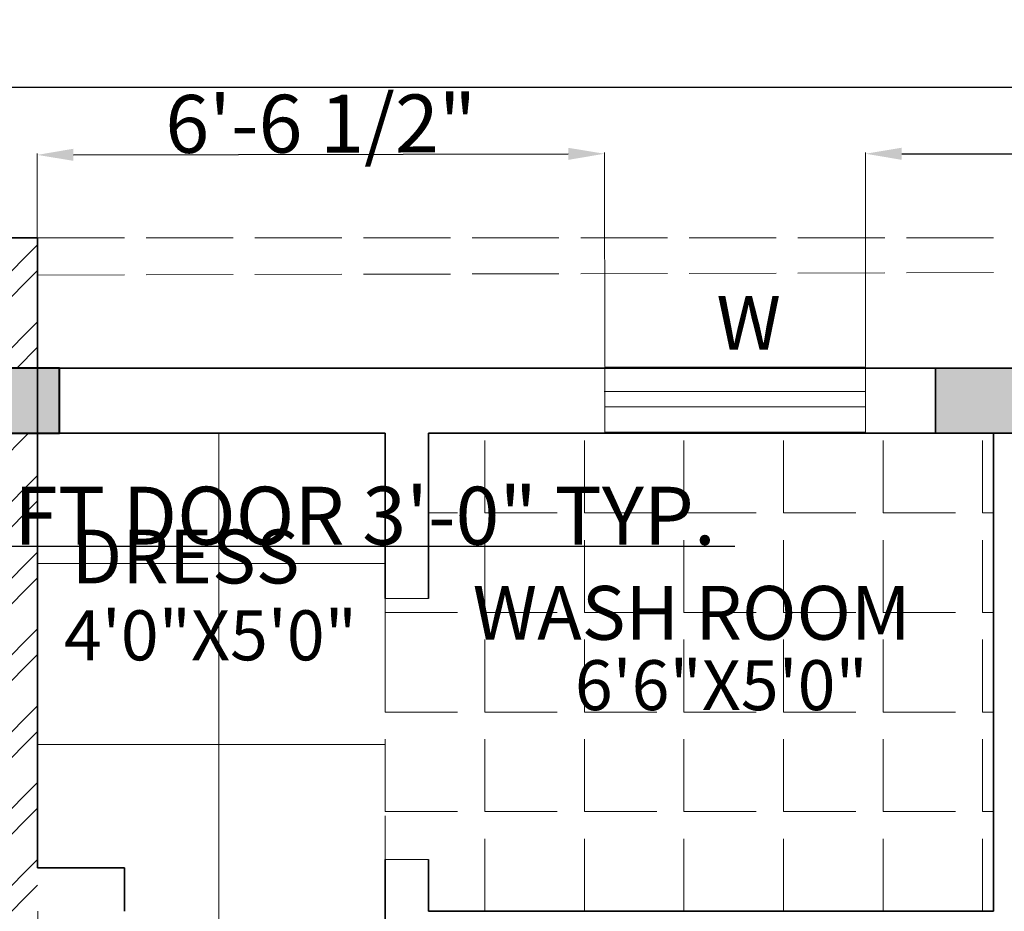
# Model space of a CAD drawing. Units: inches. Extents: x 351 to 1738, y -265 to 286.
# Tile 27 of 38: x 1110 to 1246, y 163 to 286. Entities that reach past the tile are written whole.
import ezdxf

# ---------------------------------------------------------------- set-up
doc = ezdxf.new("R2010")
doc.units = ezdxf.units.IN
doc.header["$MEASUREMENT"] = 0
doc.linetypes.add('ACAD_ISO02W100', pattern=[15, 12, -3])
doc.linetypes.add('ACAD_ISO03W100', pattern=[30, 12, -18])
for name, color, linetype, lineweight in [('A-ANNO-DIMS', 2, 'Continuous', 18), ('A-ANNO-SYMB', 7, 'Continuous', 18), ('A-AREA-IDEN', 7, 'Continuous', 18), ('A-COLS', 7, 'Continuous', 40), ('A-COLS-PATT', 6, 'Continuous', 13), ('A-DOOR', 3, 'Continuous', 18), ('A-DOOR-HIDN', 3, 'ACAD_ISO03W100', 13), ('A-FLOR-OVHD', 1, 'ACAD_ISO02W100', 18), ('A-FLOR-PATT', 9, 'Continuous', 9), ('A-GLAZ', 4, 'Continuous', 18), ('A-WALL', 7, 'Continuous', 35), ('A-WALL-PATT', 152, 'Continuous', 13)]:
    doc.layers.add(name, color=color, linetype=linetype, lineweight=lineweight)
doc.styles.add('Annotative', font='arial.ttf')
doc.styles.get("Standard").update_dxf_attribs({"font": 'arial.ttf'})
doc.dimstyles.get("Standard").update_dxf_attribs({"dimtxt": 8, "dimasz": 5, "dimexe": 0.18, "dimexo": 0.0625, "dimgap": 0.09, "dimtad": 1, "dimtoh": 1, "dimzin": 0, "dimdsep": 46, "dimlunit": 4, "dimtxsty": 'Standard', "dimcen": 0, "dimclre": 256, "dimadec": 0, "dimazin": 0, "dimtfac": 1, "dimtofl": 0, "dimtmove": 0, "dimatfit": 3, "dimfxl": 1, "dimtolj": 1, "dimtzin": 0, "dimlwe": -1, "dimarcsym": 0})

# ---------------------------------------------------------------- blocks, each defined once
blk = doc.blocks.new('*D7')
at = {"layer": 'A-ANNO-DIMS', "color": 0, "transparency": 16777216}
for p, q in [((1034.7, 256.03), (1034.7, 276.92)), ((1566.7, 256.03), (1566.7, 276.92))]:
    blk.add_line(p, q, dxfattribs=at)
at = {"layer": 'A-ANNO-DIMS', "color": 0, "lineweight": -2, "transparency": 16777216}
blk.add_line((1039.7, 276.74), (1561.7, 276.74), dxfattribs=at)
at = {"layer": 'A-ANNO-DIMS', "color": 0, "transparency": 16777216}
for points in [[(1039.7, 277.57), (1039.7, 275.91), (1034.7, 276.74)], [(1561.7, 277.57), (1561.7, 275.91), (1566.7, 276.74)]]:
    blk.add_solid(points, dxfattribs=at)
at = {"layer": 'Defpoints', "color": 0, "transparency": 16777216}
for p in [(1566.7, 276.74), (1034.7, 255.96), (1566.7, 255.96)]:
    blk.add_point(p, dxfattribs=at)
at = {"layer": 'A-ANNO-DIMS', "color": 0, "transparency": 16777216, "insert": (1300.7, 280.83), "char_height": 8, "attachment_point": 5}
blk.add_mtext('\\A1;44\'-4"', dxfattribs=at)
blk = doc.blocks.new('*D54')
at = {"layer": 'A-ANNO-DIMS', "transparency": 16777216}
for p, q in [((1056.7, 208.03), (1056.7, 213.54)), ((1092.7, 208.03), (1092.7, 213.54))]:
    blk.add_line(p, q, dxfattribs=at)
at = {"layer": 'A-ANNO-DIMS', "color": 0, "lineweight": -2, "transparency": 16777216}
for p, q in [((1061.7, 213.36), (1087.7, 213.36)), ((1092.7, 213.36), (1209.01, 213.36))]:
    blk.add_line(p, q, dxfattribs=at)
at = {"layer": 'A-ANNO-DIMS', "color": 0, "transparency": 16777216}
for points in [[(1061.7, 214.2), (1061.7, 212.53), (1056.7, 213.36)], [(1087.7, 214.2), (1087.7, 212.53), (1092.7, 213.36)]]:
    blk.add_solid(points, dxfattribs=at)
at = {"layer": 'Defpoints', "color": 0, "transparency": 16777216}
for p in [(1092.7, 213.36), (1056.7, 207.96), (1092.7, 207.96)]:
    blk.add_point(p, dxfattribs=at)
at = {"layer": 'A-ANNO-DIMS', "color": 0, "transparency": 16777216, "insert": (1153.35, 217.59), "char_height": 8, "attachment_point": 5}
blk.add_mtext('\\A1;LIFT DOOR 3\'-0" TYP.', dxfattribs=at)
blk = doc.blocks.new('*D62')
at = {"layer": 'A-ANNO-DIMS', "transparency": 16777216}
for p, q in [((1112.7, 238.03), (1112.65, 267.59)), ((1191.04, 238.18), (1190.98, 267.75))]:
    blk.add_line(p, q, dxfattribs=at)
at = {"layer": 'A-ANNO-DIMS', "color": 0, "lineweight": -2, "transparency": 16777216}
blk.add_line((1117.65, 267.42), (1185.98, 267.56), dxfattribs=at)
at = {"layer": 'A-ANNO-DIMS', "color": 0, "transparency": 16777216}
for points in [[(1117.65, 268.26), (1117.65, 266.59), (1112.65, 267.41)], [(1185.98, 268.39), (1185.98, 266.72), (1190.98, 267.57)]]:
    blk.add_solid(points, dxfattribs=at)
at = {"layer": 'Defpoints', "color": 0, "transparency": 16777216}
for p in [(1190.98, 267.57), (1191.04, 238.12), (1112.7, 237.96)]:
    blk.add_point(p, dxfattribs=at)
at = {"layer": 'A-ANNO-DIMS', "color": 0, "transparency": 16777216, "insert": (1151.81, 271.72), "char_height": 8, "attachment_point": 5, "rotation": 0.1116}
blk.add_mtext('\\A1;6\'-6 1/2"', dxfattribs=at)
blk = doc.blocks.new('*D63')
at = {"layer": 'A-ANNO-DIMS', "transparency": 16777216}
for p, q in [((1227.04, 238.18), (1227.04, 267.75)), ((1266.55, 238.18), (1266.55, 267.75))]:
    blk.add_line(p, q, dxfattribs=at)
at = {"layer": 'A-ANNO-DIMS', "color": 0, "lineweight": -2, "transparency": 16777216}
for p, q in [((1232.04, 267.57), (1261.55, 267.57)), ((1266.55, 267.57), (1311.63, 267.57))]:
    blk.add_line(p, q, dxfattribs=at)
at = {"layer": 'A-ANNO-DIMS', "color": 0, "transparency": 16777216}
for points in [[(1232.04, 268.4), (1232.04, 266.73), (1227.04, 267.57)], [(1261.55, 268.4), (1261.55, 266.73), (1266.55, 267.57)]]:
    blk.add_solid(points, dxfattribs=at)
at = {"layer": 'Defpoints', "color": 0, "transparency": 16777216}
for p in [(1266.55, 267.57), (1227.04, 238.12), (1266.55, 238.12)]:
    blk.add_point(p, dxfattribs=at)
at = {"layer": 'A-ANNO-DIMS', "color": 0, "transparency": 16777216, "insert": (1291.59, 271.79), "char_height": 8, "attachment_point": 5}
blk.add_mtext('\\A1;3\'-3 1/2"', dxfattribs=at)

msp = doc.modelspace()

# ---------------------------------------------------------------- hatches: boundary and pattern name
at = {"layer": 'A-COLS-PATT'}
h = msp.add_hatch(color=256, dxfattribs=at)
h.dxf.hatch_style = 1
h.paths.add_polyline_path([(1112.704, 237.963), (1103.704, 237.963), (1103.704, 228.963), (1112.704, 228.963)])
h.paths.add_polyline_path([(1115.704, 237.963), (1112.704, 237.963), (1112.704, 228.963), (1115.704, 228.963)])
h.paths.add_polyline_path([(1043.704, 255.963), (1034.704, 255.963), (1034.704, 243.963), (1043.704, 243.963)])
h.paths.add_polyline_path([(1043.704, 210.963), (1034.704, 210.963), (1034.704, 198.963), (1043.704, 198.963)])
h.paths.add_polyline_path([(1043.704, -45.037), (1034.704, -45.037), (1034.704, -57.037), (1043.704, -57.037)])
h.paths.add_polyline_path([(1112.704, -45.037), (1103.704, -45.037), (1103.704, -57.037), (1112.704, -57.037)])
h.paths.add_polyline_path([(1112.704, -161.037), (1103.704, -161.037), (1103.704, -164.037), (1103.704, -173.037), (1112.704, -173.037)])
h.paths.add_polyline_path([(1043.704, -161.037), (1034.704, -161.037), (1034.704, -173.037), (1043.704, -173.037)])
h.paths.add_polyline_path([(1248.549, -164.037), (1236.549, -164.037), (1236.549, -173.037), (1248.549, -173.037)])
h.paths.add_polyline_path([(1248.549, -50), (1236.549, -50), (1236.549, -59), (1248.549, -59)])
h.paths.add_polyline_path([(1248.704, 73.463), (1244.704, 73.463), (1244.704, 64.463), (1248.704, 64.463)])
h.paths.add_polyline_path([(1244.704, 73.463), (1236.704, 73.463), (1236.704, 64.463), (1244.704, 64.463)])
h.paths.add_polyline_path([(1248.704, 237.963), (1236.704, 237.963), (1236.704, 228.963), (1248.704, 228.963)])
h.paths.add_polyline_path([(1392.204, 237.963), (1380.204, 237.963), (1380.204, 228.963), (1392.204, 228.963)])
h.paths.add_polyline_path([(1536.064, 237.963), (1524.064, 237.963), (1524.064, 228.963), (1536.064, 228.963)])
h.paths.add_polyline_path([(1536.064, 73.463), (1524.064, 73.463), (1524.064, 64.463), (1536.064, 64.463)])
h.paths.add_polyline_path([(1384.204, 73.463), (1380.204, 73.463), (1380.204, 64.463), (1384.204, 64.463)])
h.paths.add_polyline_path([(1392.064, 73.463), (1384.204, 73.463), (1384.204, 64.463), (1392.064, 64.463)])
h.paths.add_polyline_path([(1536.064, -53.037), (1524.064, -53.037), (1524.064, -57.037), (1536.064, -57.037)])
h.paths.add_polyline_path([(1536.064, -48.037), (1524.064, -48.037), (1524.064, -53.037), (1536.064, -53.037)])
h.paths.add_polyline_path([(1392.064, -48.037), (1380.064, -48.037), (1380.064, -56.5), (1380.065, -57.037), (1392.064, -57.037)])
h.paths.add_polyline_path([(1536.064, -164.037), (1524.064, -164.037), (1524.064, -173.037), (1536.064, -173.037)])
at = {"layer": 'A-FLOR-PATT', "transparency": 33554559}
h = msp.add_hatch(dxfattribs=at)
h.set_pattern_fill('ANSI37', color=256, scale=200, angle=135)
h.set_pattern_definition([(180, (1112.704, -164.037), (-2e-15, -25), []), (270, (1112.704, -164.037), (25, -5e-15), [])])
h.paths.add_polyline_path([(1380.064, 73.463), (1380.132, 148.463), (1338.064, 148.463), (1290.704, 148.463), (1290.704, 88.463), (1248.704, 88.463), (1248.704, -2.009), (1244.704, -2.009), (1244.704, 142.457), (1160.704, 142.457), (1160.704, 158.963), (1160.704, 170.137), (1160.704, 206.137), (1160.704, 228.963), (1112.704, 228.963), (1112.704, 209.963), (1112.704, 168.963), (1124.704, 168.963), (1124.704, 162.963), (1112.704, 162.963), (1112.704, 64.463), (1112.704, 60.463), (1112.704, 0.463), (1112.704, -48.026), (1146.804, -47.981), (1146.804, -35.691), (1207.804, -35.691), (1207.804, -47.902), (1236.542, -47.864), (1236.544, -50.009), (1248.5, -50.009), (1248.506, -102.915), (1248.512, -150.915), (1248.514, -164.037), (1248.549, -164.037), (1273.017, -164.037), (1273.017, -128.799), (1355.24, -128.799), (1355.24, -164.037), (1384.204, -164.037), (1384.204, -57.037), (1380.064, -57.037), (1380.064, -48.037), (1392.064, -48.037), (1392.064, -53.037), (1406.549, -53.037), (1406.549, -57.037), (1401.204, -57.037), (1401.204, -147.037), (1468.204, -147.037), (1468.204, -138.5), (1472.204, -138.5), (1472.204, -102.5), (1468.204, -102.5), (1468.204, -57.037), (1442.549, -57.037), (1442.549, -53.037), (1463.049, -53.037), (1463.049, -40.747), (1524.049, -40.747), (1524.049, -48.037), (1536.064, -48.037), (1536.064, -53.037), (1557.704, -53.037), (1557.704, 204.963), (1384.204, 204.963), (1384.204, 73.463), (1392.064, 73.463), (1392.064, 64.463), (1384.204, 64.463), (1384.204, -3.5), (1380.204, -3.537), (1380.204, 64.463), (1380.064, 64.463)])
h.paths.add_polyline_path([(1510.714, 86.458, -0.1039845), (1511.661, 85.595, 0.4704384), (1510.158, 87.614, 0.0961001)], flags=16)
h.paths.add_polyline_path([(1510.443, 100.266, 0.009798), (1504.693, 100.48, 0.0287898), (1504.6, 99.767, -0.1653311), (1505.519, 96.135, -0.1436014)], flags=16)
h.paths.add_polyline_path([(1487.201, 85.595, -0.1039845), (1488.148, 86.458, 0.0961001), (1488.704, 87.614, 0.4704384)], flags=0)
h.paths.add_polyline_path([(1495.052, 100.43), (1494.178, 100.43, -0.0264629), (1494.262, 99.774, -0.1442193)], flags=16)
h.paths.add_polyline_path([(1444.485, 86.458, -0.1039845), (1445.433, 85.595, 0.4704384), (1443.93, 87.614, 0.0961001)], flags=16)
h.paths.add_polyline_path([(1420.972, 85.595, -0.1039845), (1421.92, 86.458, 0.0961001), (1422.475, 87.614, 0.4704384)], flags=16)
h.paths.add_polyline_path([(1428.632, 100.335, 0.0010541), (1427.971, 100.309, -0.0215241), (1428.033, 99.774, -0.1143008)], flags=16)
h.paths.add_polyline_path([(1419.906, 143.708, 0.0249793), (1420.222, 157.526), (1421.573, 159.101), (1421.573, 175.369), (1391.393, 175.369), (1391.393, 200.519), (1542.294, 200.519), (1542.294, 175.369), (1512.028, 175.369, 0.0198653), (1511.521, 153.838, 0.0251335), (1512.758, 118.323, 0.0205529), (1512.942, 115.253), (1419.834, 115.253, -0.0004142), (1419.843, 124.798), (1413.059, 124.798), (1413.059, 84.437, -0.0618528), (1415.831, 80.45, -0.0930773), (1420.972, 85.595, -0.2675367), (1422.371, 84.732, 0.0851103), (1424.052, 84.616, -0.8853927), (1424.033, 84.851, -1.1258145), (1424.073, 84.366, -0.0879871), (1422.371, 84.732, -0.2675367), (1422.326, 83.089, -0.3705421), (1420.972, 85.595, 0.0930773), (1415.831, 80.45, -0.0874142), (1417.914, 73.937), (1418.941, 73.937, 0.0272504), (1418.913, 76.906, -0.1157032), (1421.051, 73.937), (1445.354, 73.937, -0.1157032), (1447.492, 76.906, 0.0272504), (1447.464, 73.937), (1448.491, 73.937, -0.0874142), (1450.574, 80.45, 0.0930773), (1445.433, 85.595, -0.3705421), (1444.079, 83.089, -0.2675367), (1444.034, 84.732, -0.0879871), (1442.332, 84.366, -1.1258145), (1442.372, 84.851, -2.0327363), (1442.364, 84.368, 0.0863779), (1444.034, 84.732, -0.2675367), (1445.433, 85.595, -0.0930773), (1450.574, 80.45, -0.2577317), (1466.483, 90.927, -0.4786702), (1468.832, 91.907, -0.4786702), (1471.18, 90.927, -0.26264), (1483.053, 81.78, -0.0718662), (1487.201, 85.595, -0.2675367), (1488.6, 84.732, 0.0851103), (1490.28, 84.616, -0.8853927), (1490.262, 84.851, -1.1258145), (1490.301, 84.366, -0.0879871), (1488.6, 84.732, -0.2675367), (1488.554, 83.089, -0.3705421), (1487.201, 85.595, 0.0718662), (1483.053, 81.78, -0.1320648), (1484.143, 73.937), (1485.169, 73.937, 0.0272504), (1485.142, 76.906, -0.1157032), (1487.28, 73.937), (1511.582, 73.937, -0.1157032), (1513.72, 76.906, 0.0272504), (1513.693, 73.937), (1514.719, 73.937, -0.0874142), (1516.802, 80.45, 0.0930773), (1511.661, 85.595, -0.3705421), (1510.308, 83.089, -0.2675367), (1510.262, 84.732, -0.0879871), (1508.561, 84.366, -1.1258145), (1508.601, 84.851, -2.0327363), (1508.592, 84.368, 0.0863779), (1510.262, 84.732, -0.2675367), (1511.661, 85.595, -0.0930773), (1516.802, 80.45, -0.0618528), (1519.575, 84.437), (1519.575, 73.937), (1413.059, 73.937), (1413.059, 124.798), (1419.843, 124.798, -0.0008205)], flags=16)
h.paths.add_polyline_path([(1220.149, 54.133, -0.1039845), (1220.869, 53.476, 0.4704384), (1219.727, 55.011, 0.0961001)], flags=16)
h.paths.add_polyline_path([(1219.944, 64.626, 0.009798), (1215.574, 64.789, 0.0287898), (1215.503, 64.247, -0.1653311), (1216.201, 61.487, -0.1436014)], flags=16)
h.paths.add_polyline_path([(1209.779, 64.449, 0.0974459), (1209.339, 64.751), (1208.247, 64.751, 0.1273905), (1207.7, 64.326, 0.1715858), (1206.95, 61.475, -0.1588542), (1207.636, 59.45, 0.0158984), (1207.795, 59.218, 0.0615457), (1208.598, 59.616, 0.1754158), (1208.638, 60.099, -0.2847793), (1209.348, 62.472, 0.3262165)], flags=16)
h.paths.add_polyline_path([(1169.818, 54.133, -0.1039845), (1170.538, 53.476, 0.4704384), (1169.396, 55.011, 0.0961001)], flags=16)
h.paths.add_polyline_path([(1159.017, 62.472, 0.2847642), (1158.307, 60.099, -0.1754332), (1158.267, 59.616, 0.3929302), (1159.448, 64.449, -0.3262298)], flags=16)
h.paths.add_polyline_path([(1156.342, 58.239, -0.1783213), (1154.011, 55.31, -0.1747359), (1154.722, 55.233, -0.2008015), (1156.27, 56.086, 0.1269899), (1157.283, 58.991, -0.0912053)], flags=16)
h.paths.add_polyline_path([(1156.624, 61.413, 0.1572752), (1157.316, 64.247, 0.1696217)], flags=16)
h.paths.add_polyline_path([(1152.67, 54.133, -0.0961001), (1151.95, 53.476, 0.0640762), (1154.465, 54.384, 0.1990158)], flags=16)
h.paths.add_polyline_path([(1202.281, 53.476, -0.1039845), (1203, 54.133, 0.0961001), (1203.423, 55.011, 0.4704384)], flags=0)
h.paths.add_polyline_path([(1151.139, 97.64, 0.0249793), (1151.379, 108.141), (1152.406, 109.338), (1152.406, 121.701), (1129.47, 121.701), (1129.47, 140.814), (1244.149, 140.814), (1244.149, 121.701), (1221.148, 121.701, 0.0198653), (1220.763, 105.338, 0.0251335), (1221.703, 78.349, 0.0205529), (1221.843, 76.016), (1151.078, 76.016, -0.1287433), (1148.786, 65.037, 0.5393525), (1150.327, 64.171, -0.027594), (1163.481, 64.751, 0.0976954), (1163.04, 64.449, 0.3262165), (1163.471, 62.472, -0.2847765), (1164.181, 60.099, -0.1947567), (1165.846, 61.443, -0.1554021), (1165.172, 64.247, -0.1660224), (1165.869, 61.475, -0.1770142), (1167.852, 62.77, -0.4482027), (1169.974, 60.807, -0.3934987), (1167.679, 57.86, -0.8955483), (1168.438, 54.524, -0.3557668), (1166.218, 56.086, -0.066024), (1165.505, 57.539), (1165.251, 56.243, -0.3717324), (1164.02, 59.758, -0.3736141), (1163.04, 64.449, -0.0976954), (1163.481, 64.751, 0.0213538), (1153.294, 64.429, -0.1341826), (1156.695, 61.368, 0.1868727), (1154.636, 62.77, 0.4482027), (1152.514, 60.807, 0.4037263), (1154.905, 57.846, 0.7112192), (1153.334, 55, 0.5315397), (1151.95, 53.476, -0.2675367), (1153.013, 52.821, 0.0851103), (1154.29, 52.732, -0.8853927), (1154.276, 52.911, -1.1258145), (1154.306, 52.543, -0.0879871), (1153.013, 52.821, -0.2675367), (1152.978, 51.572, -0.3705421), (1151.95, 53.476, 0.0930773), (1148.043, 49.566, -0.0874142), (1149.626, 44.617), (1150.406, 44.617, 0.0272504), (1150.385, 46.873, -0.1157032), (1152.01, 44.617), (1170.478, 44.617, -0.1157032), (1172.103, 46.873, 0.0272504), (1172.082, 44.617), (1172.862, 44.617, -0.0874142), (1174.445, 49.566, 0.0930773), (1170.538, 53.476, -0.3705421), (1169.51, 51.572, -0.2675367), (1169.475, 52.821, -0.0879871), (1168.182, 52.543, -1.1258145), (1168.212, 52.911, -2.0327363), (1168.206, 52.544, 0.0863779), (1169.475, 52.821, -0.2675367), (1170.538, 53.476, -0.0930773), (1174.445, 49.566, -0.2577317), (1186.536, 57.528, -0.4786702), (1188.321, 58.273, -0.4786702), (1190.106, 57.528, -0.26264), (1199.128, 50.577, -0.0718662), (1202.281, 53.476, -0.2675367), (1203.344, 52.821, 0.0851103), (1204.621, 52.732, -0.8853927), (1204.607, 52.911, -1.1258145), (1204.637, 52.543, -0.0879871), (1203.344, 52.821, -0.2675367), (1203.309, 51.572, -0.3705421), (1202.281, 53.476, 0.0718662), (1199.128, 50.577, -0.1320648), (1199.957, 44.617), (1200.737, 44.617, 0.0272504), (1200.716, 46.873, -0.1157032), (1202.341, 44.617), (1220.809, 44.617, -0.1157032), (1222.434, 46.873, 0.0272504), (1222.413, 44.617), (1223.193, 44.617, -0.0874142), (1224.776, 49.566, 0.0930773), (1220.869, 53.476, -0.3705421), (1219.841, 51.572, -0.2675367), (1219.806, 52.821, -0.0879871), (1218.513, 52.543, -1.1258145), (1218.543, 52.911, -2.0327363), (1218.537, 52.544, 0.0863779), (1219.806, 52.821, -0.2675367), (1220.869, 53.476, -0.0930773), (1224.776, 49.566, -0.0618528), (1226.883, 52.597), (1226.883, 44.617), (1145.936, 44.617), (1145.936, 83.269), (1151.091, 83.269, -0.0008205)], flags=16)
h.paths.add_polyline_path([(1218.01, 57.86, -0.8955483), (1218.769, 54.524, -0.3557668), (1216.549, 56.086, -0.066024), (1215.836, 57.539), (1215.582, 56.243, -0.3717324), (1214.351, 59.758, -0.3736141), (1213.371, 64.449, 0.3262165), (1213.802, 62.472, -0.2847765), (1214.512, 60.099, -0.1947567), (1216.177, 61.443, -0.1799907), (1218.183, 62.77, -0.4482027), (1220.305, 60.807, -0.3934987)], flags=16)
h.paths.add_polyline_path([(1424.735, 91.363, -0.3934987), (1421.715, 95.241, -0.4482027), (1424.507, 97.824, -0.1799907), (1427.147, 96.077, -0.1947567), (1429.338, 94.309, -0.2847765), (1430.272, 97.432, 0.3262165), (1430.839, 100.034, -0.3736141), (1429.55, 93.861, -0.3717324), (1427.929, 89.235), (1427.596, 90.941, -0.066024), (1426.657, 89.029, -0.3557668), (1423.736, 86.973, -0.8955483)], flags=16)
h.paths.add_polyline_path([(1238.033, 131.257, -1), (1227.329, 131.257, -1)], flags=0)
h.paths.add_polyline_path([(1235.357, 131.257, -1), (1230.005, 131.257, -1)], flags=0)
h.paths.add_polyline_path([(1214.039, 54.243, 0.1543819), (1214.38, 53.992, 0.3589549), (1213.613, 54.016, 0.6039484), (1214.379, 53.657, 0.3713191), (1213.968, 52.872, 0.1879935), (1214.312, 52.809, -0.592455), (1213.953, 52.967, -0.2942791), (1214.083, 53.691, -1.3001871), (1213.881, 54.134, -0.2837621), (1214.469, 53.896, 1.1509396)], flags=16)
h.paths.add_polyline_path([(1212.091, 56.286, -0.4084338), (1211.337, 56.445, -0.0362594), (1211.098, 56.848, -0.2360976), (1211.59, 56.63, 0.0353445), (1211.835, 56.543, -0.4752408), (1212.091, 56.286, -0.4752408), (1212.438, 56.182, 0.0353445), (1212.631, 56.007, -0.2360976), (1213.056, 55.676, -0.0362594), (1212.588, 55.697, -0.4084338)], flags=16)
h.paths.add_polyline_path([(1211.469, 50.297, 0.296043), (1210.47, 50.527, 0.310883), (1211.931, 50.148, 0.0212546)], flags=16)
h.paths.add_polyline_path([(1213.739, 51.818, -0.0362594), (1213.271, 51.838, -0.4084337), (1212.774, 52.427, -0.0947856), (1212.293, 50.703, 1.1504738), (1212.911, 50.232, 0.1662877), (1213.265, 50.68, -0.0252543), (1212.603, 50.13, 1.0879317), (1212.471, 49.407, 0.1662877), (1213.02, 49.251, -0.016128), (1212.567, 49.563, -0.286859), (1212.217, 49.638, 0.0221563), (1212.046, 50.055, -0.6461302), (1212.185, 50.498, 0.0884116), (1212.732, 52.077, -1.1860374), (1213.121, 52.323, 0.0353445), (1213.314, 52.148, -0.2360976)], flags=16)
h.paths.add_polyline_path([(1212.094, 50.342, -0.0485241), (1211.54, 49.605, -1.1038339), (1211.397, 48.738, -0.7855147), (1211.683, 48.254, -0.3920429), (1210.948, 48.525, -0.3928194), (1210.561, 47.995, -0.592455), (1210.201, 48.153, -0.2942791), (1210.331, 48.877, -0.7041716), (1210.316, 49.592, -0.6793441), (1210.729, 50.112, 0.5636764)], flags=16)
h.paths.add_polyline_path([(1211.274, 49.829, -0.1398258), (1210.745, 49.859, -0.2178785), (1210.948, 49.509, -0.4985724)], flags=0)
h.paths.add_polyline_path([(1433.426, 81.49, -0.181571), (1434.245, 81.788, -0.0080665), (1433.726, 82.205, 0.0455784), (1432.755, 81.242, 0.1790113)], flags=16)
h.paths.add_polyline_path([(1434.146, 81.009, -0.1324418), (1433.645, 80.771, 0.2590893), (1433.234, 80.471, -0.1802109), (1433.392, 80.805, -0.1699398), (1432.758, 81.109, 0.0326525), (1433.273, 80.474, -0.4933627), (1434.046, 80.146, -0.3904966)], flags=16)
h.paths.add_polyline_path([(1434.83, 80.047, -0.9475376), (1435.294, 79.576, -0.2991282), (1434.625, 79.404, -0.2704392), (1435.01, 78.591, -0.592455), (1434.537, 78.382, -0.3928194), (1434.027, 79.08, -0.3920429), (1433.06, 78.723, -0.3520423), (1433.003, 79.197, -0.1972159), (1433.75, 79.734, -0.7136405), (1434.447, 79.939, -0.2147903), (1434.819, 80.475, 0.4088333), (1435.075, 80.803, -0.2261519)], flags=16)
h.paths.add_polyline_path([(1432.67, 81.217, -0.4542182), (1431.897, 79.923, -0.4144105), (1431.301, 80.035, 0.0161291), (1431.897, 80.445, 0.2795702), (1432.073, 80.871, -0.2895037), (1431.103, 81.321, -0.4144105), (1430.978, 81.915, 0.0161296), (1431.586, 81.521, 0.341293), (1432.125, 81.583, -0.8131856)], flags=16)
h.paths.add_polyline_path([(1429.893, 86.381, -0.9475376), (1430.358, 85.91, -0.1731062), (1429.984, 85.712, -0.0388172), (1431.625, 84.214, -0.0879005), (1432.097, 88.549, -0.0497684), (1431.254, 88.49, -0.2360976), (1431.814, 88.925, 0.0353445), (1432.067, 89.155, -0.4752408), (1432.524, 89.291, -0.4752408), (1432.86, 89.63, 0.0353445), (1433.182, 89.744, -0.2360976), (1433.83, 90.032, -0.0362594), (1433.516, 89.502, -0.4084338), (1432.524, 89.291, -0.3124239), (1432.106, 88.58, 0.0885594), (1431.625, 84.214, -0.4084337), (1430.971, 83.439, -0.0362594), (1430.355, 83.412, -0.2360976), (1430.914, 83.847, 0.0353445), (1431.168, 84.078, -0.4752408), (1431.625, 84.214, 0.0388172), (1429.984, 85.712, -0.3217316), (1429.333, 86.048, -0.32743), (1429.883, 86.809, 0.4088333), (1430.138, 87.138, -0.2261519)], flags=16)
h.paths.add_polyline_path([(1211.206, 58.616, -0.9997836), (1211.336, 59.323, -0.6149935)], flags=16)
h.paths.add_polyline_path([(1210.288, 49.429, 0.1543819), (1210.629, 49.178, 0.3589549), (1209.861, 49.202, 0.6039484), (1210.627, 48.843, -0.5348247), (1210.806, 49.295, 0.7483464)], flags=16)
h.paths.add_polyline_path([(1209.589, 51.828, -0.0087906), (1209.775, 51.753, 0.1122315), (1209.466, 52.019, 1.4188509), (1209.014, 51.708, -0.4587257), (1208.651, 51.073, -0.592455), (1208.291, 51.232, -0.2942791), (1208.421, 51.955, -1.3001871), (1208.219, 52.398, -0.2260052), (1208.719, 52.257, -0.4755189), (1209.158, 52.369, -1.4554994), (1209.603, 52.664, 0.4213049), (1209.191, 52.262, -0.5912116), (1208.979, 51.796, 0.4973986), (1209.773, 51.333, 0.6493116)], flags=16)
h.paths.add_polyline_path([(1208.029, 52.041, 0.5446671), (1208.832, 52.045, 0.220132)], flags=0)
h.paths.add_polyline_path([(1210.438, 51.425, -0.2041997), (1210.277, 52.018, 0.2708262), (1209.915, 52.897, 0.3241145)], flags=0)
h.paths.add_polyline_path([(1209.668, 52.407, -0.60139), (1208.99, 52.221, -0.3949159), (1208.248, 52.83, -0.8367916), (1208.651, 53.017, -0.3384876), (1209.039, 52.571, 0.1941379), (1209.191, 52.262, 0.4139945), (1209.712, 52.475, 0.5177103), (1210.503, 51.416, 0.401922), (1209.493, 50.93, 0.2063956), (1209.516, 50.165, -0.3194629), (1210.417, 51.418, -0.466635)], flags=16)
h.paths.add_polyline_path([(1206.601, 56.086, -0.3557668), (1204.381, 54.524, -0.9211983), (1205.236, 57.846, 0.2065693), (1207.614, 58.991, -0.1269899)], flags=16)
h.paths.add_polyline_path([(1435.487, 82.816, 0.5277653), (1436.615, 83.361, 0.5085402), (1437.05, 82.433, 0.592455), (1437.524, 82.641, 0.3312448), (1436.963, 83.548, 0.3878632), (1437.808, 83.626, 0.5929544), (1437.618, 84.176, 0.2260158), (1436.961, 83.99, 0.3182053), (1437.588, 84.854, 0.6893744), (1437.05, 84.991, 0.3357648), (1436.539, 84.41, -0.1569934), (1436.404, 84.065, -0.4346112), (1436.961, 83.99, -0.2147903), (1437.333, 84.526, 0.4088333), (1437.588, 84.854, -0.2261519), (1437.343, 84.097, -0.9475376), (1437.808, 83.626, -0.2991282), (1437.139, 83.455, -0.2704392), (1437.524, 82.641, -0.592455), (1437.05, 82.433, -0.3928194), (1436.541, 83.13, -0.4396601), (1435.475, 82.794, -0.174614), (1435.942, 82.244, -0.2063956), (1435.912, 81.237, -0.2708262), (1435.125, 82.208, 0.2079765), (1434.686, 82.904, -0.1964955)], flags=16)
h.paths.add_polyline_path([(1435.386, 84.832, 0.270811), (1434.91, 83.676, -0.2042174), (1434.699, 82.895, 0.3241145)], flags=0)
h.paths.add_polyline_path([(1435.68, 84.18, -0.2176564), (1435.554, 83.304, -0.1767045), (1436.236, 83.778, -0.3730364)], flags=0)
h.paths.add_polyline_path([(1435.566, 100.034, 0.3262165), (1436.133, 97.432, -0.2847765), (1437.067, 94.309, -0.1947567), (1439.258, 96.077, -0.1554021), (1438.371, 99.767, -0.1660224), (1439.289, 96.12, -0.1770142), (1441.897, 97.824, -0.4482027), (1444.69, 95.241, -0.3934987), (1441.67, 91.363, -0.8955483), (1442.669, 86.973, -0.3557668), (1439.748, 89.029, -0.066024), (1438.809, 90.941), (1438.476, 89.235, -0.3717324), (1436.855, 93.861, -0.3736141)], flags=16)
h.paths.add_polyline_path([(1191.252, 49.507, -0.2740221), (1190.658, 48.409, 0.2675367), (1191.311, 47.344, 0.3705421)], flags=0)
h.paths.add_polyline_path([(1190.301, 49.717, 0.1990158), (1188.619, 49.04, 0.0640762), (1191.252, 49.507, -0.0961001)], flags=0)
h.paths.add_polyline_path([(1189.518, 47.857, 1.1258145), (1189.676, 47.523, 2.0446052)], flags=0)
h.paths.add_polyline_path([(1464.974, 80.372, 0.2740221), (1465.756, 78.927, -0.0830131)], flags=0)
h.paths.add_polyline_path([(1464.974, 80.372, 0.3705421), (1464.897, 77.525, 0.5763244)], flags=0)
h.paths.add_polyline_path([(1464.974, 80.372, -0.4704384), (1467.284, 81.372, -0.0961001), (1466.226, 80.648, -0.1990158), (1468.439, 79.757, -0.0640762)], flags=0)
h.paths.add_polyline_path([(1189.511, 56.43, -0.2594668), (1188.321, 56.391, -0.2594668), (1187.13, 56.43, 0.0851103), (1188.193, 55.716, -0.8853927), (1188.27, 55.878, -1.1960133), (1188.355, 55.442, 0.1014587)], flags=0)
h.paths.add_polyline_path([(1188.321, 57.596, 0.0780722), (1187.678, 57.24, 0.0155503), (1188.321, 57.136, 0.0155503), (1188.964, 57.24, 0.0780722)], flags=0)
h.paths.add_polyline_path([(1190.164, 55.365, -0.5763244), (1190.106, 57.528, -0.1982945), (1188.321, 58.319, -0.1982945), (1186.536, 57.528, -0.5763244), (1186.477, 55.365, -0.3705421), (1186.536, 57.528, 0.1982945), (1188.321, 58.319, 0.1982945), (1190.106, 57.528, -0.3705421)], flags=0)
h.paths.add_polyline_path([(1188.372, 55.878, 1.1258145), (1188.529, 55.544, 2.0446052)], flags=0)
h.paths.add_polyline_path([(1186.341, 49.717, -0.0961001), (1185.389, 49.507, 0.0640762), (1188.022, 49.04, 0.1990158)], flags=0)
h.paths.add_polyline_path([(1185.389, 49.507, -0.2675367), (1185.984, 48.409, 0.0851103), (1187.046, 47.695, -0.8853927), (1187.123, 47.857, -1.1258145), (1186.966, 47.523, -0.0879871), (1185.984, 48.409, -0.2675367), (1185.331, 47.344, -0.3705421)], flags=0)
h.paths.add_polyline_path([(1399.441, 187.944, -1), (1413.525, 187.944, -1)], flags=0)
h.paths.add_polyline_path([(1402.962, 187.944, -1), (1410.004, 187.944, -1)], flags=0)
h.paths.add_polyline_path([(1357.663, -72.245), (1377.272, -72.245), (1377.272, -91.854), (1357.663, -91.854)], flags=16)
h.paths.add_polyline_path([(1467.256, 78.201, -1.1258145), (1467.049, 77.761, -2.0446052)], flags=0)
h.paths.add_polyline_path([(1468.822, 88.714, 0.9411249), (1469.106, 88.316, 1.1371523), (1468.765, 88.755, 0.890986), (1468.99, 88.245, 0.0948283), (1470.398, 89.481, -0.2675367), (1471.18, 90.927, -0.0281232), (1469.678, 90.547, -0.0287737), (1469.948, 90.311, -0.0203267), (1468.832, 90.41, -0.0203267), (1467.716, 90.311, -0.0287737), (1467.986, 90.547, -0.0281232), (1466.483, 90.927, -0.2675367), (1467.265, 89.481, 0.0851103), (1468.663, 88.542, -1.2023159)], flags=0)
h.paths.add_polyline_path([(1178.25, 124.523, -0.1199286), (1165.65, 124.145, -0.1073492), (1159.133, 124.446, -0.1028906), (1159.132, 130.465, -0.0748968), (1158.993, 137.956, 0.002027), (1167.844, 137.479, -0.07553), (1180.337, 137.666, -0.0758613), (1186.502, 137.688, -0.1409896), (1186.272, 130.046, -0.0954805), (1186.729, 124.748, -0.10603)], flags=0)
h.paths.add_polyline_path([(1469.225, 79.757, -0.1990158), (1471.437, 80.648, -0.0961001), (1470.379, 81.372, -0.4704384), (1472.689, 80.372, -0.3705421), (1472.766, 77.525, -0.2675367), (1471.907, 78.927, -0.0879863), (1470.615, 77.761, -1.1258491), (1470.408, 78.201, -2.0327363), (1470.642, 77.778, 0.0863779), (1471.907, 78.927, -0.2675367), (1472.689, 80.372, -0.0640762)], flags=0)
h.paths.add_polyline_path([(1430.423, 186.902, -0.0748968), (1430.24, 196.758, 0.002027), (1441.887, 196.131, -0.07553), (1458.326, 196.377, -0.0758613), (1466.438, 196.406, -0.1409896), (1466.136, 186.35, -0.0954805), (1466.737, 179.378, -0.10603), (1455.58, 179.082, -0.1199286), (1439, 178.585, -0.1073492), (1430.425, 178.981, -0.1028906)], flags=0)
h.paths.add_polyline_path([(1162.258, 49.939, 0.3357645), (1161.87, 49.497, -0.1569936), (1161.767, 49.235, -0.4346112), (1162.19, 49.178, -0.2147903), (1162.473, 49.585, 1.5291948)], flags=16)
h.paths.add_polyline_path([(1161.683, 49.021, 0.5815181), (1161.268, 49.583, 0.5927609)], flags=16)
h.paths.add_polyline_path([(1162.602, 48.058, 0.3713191), (1162.192, 48.843, 0.4345332), (1162.88, 48.962, 0.1850806), (1162.197, 48.926, 1.1218369)], flags=16)
h.paths.add_polyline_path([(1161.443, 48.941, -1.3071038), (1161.495, 48.571, -0.2177521), (1161.136, 48.254, 0.6973029), (1161.871, 49.048, 0.1215141)], flags=16)
h.paths.add_polyline_path([(1162.531, 49.429, -0.2070837), (1162.05, 49.146, -0.9920299)], flags=16)
h.paths.add_polyline_path([(1161.304, 49.578, -0.7196675), (1161.513, 50.079, -0.1304275), (1160.836, 50.168, 0.0395926)], flags=0)
h.paths.add_polyline_path([(1162.036, 50.584, -0.0080665), (1161.642, 50.9, 0.0293675), (1161.35, 50.297, -0.2057884)], flags=16)
h.paths.add_polyline_path([(1162.882, 51.392, -0.1247327), (1162.763, 51.828, -0.1011907), (1162.399, 51.438, -0.153425)], flags=0)
h.paths.add_polyline_path([(1164.235, 51.85, -0.3091075), (1164.513, 51.136, -0.6271245), (1163.781, 51.603, -0.6859091), (1162.777, 51.219, -0.2332851), (1163.303, 50.165, -0.2708262), (1162.705, 50.903, 0.2041997), (1162.381, 51.425, 0.204182), (1162.542, 52.018, -0.2708414), (1162.903, 52.897, -0.1272607), (1163.219, 52.529, -1.1686811), (1163.781, 52.587, -0.3291117), (1164.168, 53.017, -0.8367917), (1164.571, 52.83, -0.1933406), (1164.391, 52.338, -0.9475376), (1164.744, 51.981, -0.2991282)], flags=16)
h.paths.add_polyline_path([(1163.598, 51.937, -1.2629561), (1163.236, 51.831, 0.0125754), (1162.971, 51.721, 0.2306566), (1163.151, 52.407, -0.1648982), (1163.178, 52.661, -0.4493201), (1163.628, 52.262, -0.721477), (1164.154, 52.088, -0.8499982)], flags=0)
h.paths.add_polyline_path([(1161.613, 58.616, -0.9804131), (1161.525, 59.049, -2.9089348)], flags=16)
h.paths.add_polyline_path([(1160.252, 49.166, -0.4144105), (1159.799, 49.251, 0.0161291), (1160.252, 49.563, 0.2795702), (1160.386, 49.887, -0.2895037), (1159.649, 50.229, -0.4144105), (1159.554, 50.68, 0.0161296), (1160.015, 50.381, 0.6178854), (1160.526, 50.703, -0.0947856), (1160.045, 52.427, -0.1404436), (1159.682, 52.042, -0.0578559), (1159.3, 51.872, 0.5448433), (1160.046, 52.419, -0.0881216), (1160.404, 55.721, -0.0497684), (1159.763, 55.676, -0.2360976), (1160.188, 56.007, 0.0353445), (1160.381, 56.182, -0.4752408), (1160.728, 56.286, -0.4752408), (1160.984, 56.543, 0.0353445), (1161.229, 56.63, -0.2360976), (1161.721, 56.848, -0.0362594), (1161.482, 56.445, -0.4084338), (1160.728, 56.286, -0.3124239), (1160.411, 55.745, 0.0885594), (1160.045, 52.427, 0.1070813), (1160.634, 50.498, -0.4947977), (1160.839, 50.149, -0.4542182)], flags=16)
h.paths.add_polyline_path([(1160.666, 49.808, -2.0765276), (1160.828, 50.172, 0.0195861)], flags=0)
h.paths.add_polyline_path([(1158.439, 53.992, 0.1543819), (1158.78, 54.243, 0.7483463), (1158.262, 54.109, -0.3382251), (1158.492, 53.839, -0.1708158), (1159.124, 53.779, 0.4957286), (1158.938, 54.134, 0.2260157)], flags=16)
h.paths.add_polyline_path([(1160.045, 52.427, 0.0388172), (1158.798, 53.565, -0.1198178), (1158.574, 53.586, -0.3091075), (1158.851, 52.872, -0.1879935), (1158.506, 52.809, 0.592455), (1158.866, 52.967, 0.3312448), (1158.44, 53.657, 0.2012451), (1158.798, 53.565, -0.034023), (1159.901, 52.578, -0.0442527), (1159.698, 52.323, -0.4752408)], flags=16)
h.paths.add_polyline_path([(1336.926, -95.392), (1336.926, -117.945), (1291.82, -117.945), (1291.82, -95.392)], flags=16)
h.paths.add_polyline_path([(1357.535, -97.244), (1357.726, -96.697, 0.0348443)], flags=16)
h.paths.add_polyline_path([(1376.693, -96.478), (1377.301, -96.5, 0.0314968), (1375.907, -96.424), (1357.726, -96.424)], flags=16)
h.paths.add_polyline_path([(1379.403, -119.667, 0.0267056), (1380.043, -119.439, -0.0152991)], flags=16)
h.paths.add_polyline_path([(1357.726, -120.202), (1357.821, -120.202), (1357.821, -120.201)], flags=16)
h.paths.add_polyline_path([(1354.171, -104.592), (1354.469, -98.672, 0.0111377)], flags=16)
h.paths.add_polyline_path([(1355.058, -119.136), (1354.578, -118.539, 0.1431635)], flags=16)
h.paths.add_polyline_path([(1378.851, -96.821), (1378.85, -96.82), (1378.85, -96.82, -0.0496798), (1380.055, -97.191), (1378.85, -96.82, 0.1500541), (1375.135, -97.188), (1375.136, -119.44, -0.0099698), (1374.747, -116.649), (1357.726, -116.649, 0.1693849), (1357.535, -119.382), (1357.535, -119.382), (1357.535, -119.382, 0.0348176), (1357.726, -119.928), (1357.726, -119.928), (1357.726, -119.929, -0.0348772), (1357.535, -119.382), (1355.507, -119.382), (1355.317, -119.278), (1357.535, -119.382, -0.1693939), (1357.726, -116.649, -0.0391513), (1374.686, -116.113, -0.0020149), (1374.625, -115.546, 0.1153223), (1369.915, -115.474, 0.0609215), (1369.922, -101.154, 0.1151459), (1374.625, -101.079, -0.0020164), (1374.686, -100.513, -0.0391511), (1357.726, -99.977), (1374.747, -99.977, -0.0099633), (1375.135, -97.188), (1375.135, -97.188, -0.1501081)], flags=16)
h.paths.add_polyline_path([(1490.963, 91.363, -0.3934987), (1487.944, 95.241, -0.4482027), (1490.736, 97.824, -0.1799907), (1493.376, 96.077, -0.1947567), (1495.567, 94.309, -0.2847765), (1496.501, 97.432, 0.3262165), (1497.068, 100.034, -0.3736141), (1495.778, 93.861, -0.3717324), (1494.158, 89.235), (1493.824, 90.941, -0.066024), (1492.886, 89.029, -0.3557668), (1489.964, 86.973, -0.8955483)], flags=16)
h.paths.add_polyline_path([(1354.86, -97.658), (1355.316, -97.348, 0.1019112)], flags=16)
h.paths.add_polyline_path([(1497.063, 83.327, 0.1767244), (1496.37, 83.785, -0.4051388), (1496.016, 83.384, 0.4973986), (1497.06, 82.774, 0.6493116), (1496.818, 83.426, -0.0087906)], flags=16)
h.paths.add_polyline_path([(1496.339, 83.783, 0.5927609), (1496.886, 84.522, 0.5815181)], flags=16)
h.paths.add_polyline_path([(1495.11, 82.641, 0.592455), (1495.583, 82.433, 0.6769152), (1495.805, 83.59, 0.3756693)], flags=16)
h.paths.add_polyline_path([(1495.015, 84.176, -0.145057), (1495.301, 84.526, -0.4088333), (1495.045, 84.854, 0.2206292), (1495.381, 84.152, -0.199594), (1495.851, 83.764, -0.5240172), (1494.826, 83.626, -0.5929976)], flags=16)
h.paths.add_polyline_path([(1501.655, 81.915, -0.0161291), (1501.048, 81.521, -0.3927187), (1500.462, 81.37, -0.2106699), (1500.607, 81.142, 0.3066994)], flags=16)
h.paths.add_polyline_path([(1500.11, 89.291, -0.4084338), (1499.118, 89.502, -0.0362594), (1498.803, 90.032, -0.2360976), (1499.451, 89.744, 0.0353445), (1499.774, 89.63, -0.4752408), (1500.11, 89.291, -0.4752408), (1500.567, 89.155, 0.0353445), (1500.82, 88.925, -0.2360976), (1501.379, 88.49, -0.0362594), (1500.763, 88.516, -0.4084338)], flags=16)
h.paths.add_polyline_path([(1498.908, 82.205, -0.0513217), (1500.013, 81.134, -0.5879306), (1500.234, 81.676, 0.1070813), (1501.009, 84.214, -0.03529)], flags=16)
h.paths.add_polyline_path([(1496.93, 83.875, -0.2063956), (1497.247, 84.832, -0.2708262), (1497.724, 83.676, 0.2079765), (1497.944, 82.884, -0.3814554)], flags=16)
h.paths.add_polyline_path([(1496.721, 81.237, 0.2708125), (1497.509, 82.208, -0.2042157), (1497.935, 82.895, 0.3241145)], flags=16)
h.paths.add_polyline_path([(1497.529, 80.125, -0.145057), (1497.814, 80.475, -0.703182), (1498.282, 81.178, -0.1229248), (1497.977, 81.714, -0.2708368), (1499.207, 81.49, 0.2079641), (1499.993, 81.248, -0.2651454), (1499.278, 80.472, 0.3819006), (1498.808, 79.947, -0.3059049), (1498.848, 79.519, 0.4994816), (1498.574, 79.217, -0.4587257), (1498.097, 78.382, -0.592455), (1497.624, 78.591, -0.2704392), (1498.009, 79.404, -0.299116), (1497.34, 79.576, -0.5930157)], flags=16)
h.paths.add_polyline_path([(1500.736, 79.923, 0.4144105), (1501.333, 80.035, -0.3216484), (1500.192, 80.765, 0.0198856), (1499.976, 81.251, 0.4653307)], flags=16)
h.paths.add_polyline_path([(1501.009, 84.214, -0.0388172), (1502.649, 85.712, -0.1730946), (1502.276, 85.91, -0.5930157), (1502.465, 86.46, -0.145057), (1502.751, 86.809, -0.4088333), (1502.495, 87.138, 0.2206292), (1502.831, 86.436, -0.199594), (1503.301, 86.048, -0.3217316), (1502.649, 85.712, 0.0388172), (1501.009, 84.214, 0.1224486), (1501.412, 83.755, 0.4754908), (1501.335, 84.226, 0.055822), (1501.719, 83.847, -0.2360976), (1502.278, 83.412, -0.0362594), (1501.663, 83.439, -0.4084338)], flags=16)
h.paths.add_polyline_path([(1501.794, 100.034, 0.3262165), (1502.362, 97.432, -0.2847765), (1503.295, 94.309, -0.1947567), (1505.486, 96.077, -0.1799907), (1508.126, 97.824, -0.4482027), (1510.918, 95.241, -0.3934987), (1507.899, 91.363, -0.8955483), (1508.898, 86.973, -0.3557668), (1505.976, 89.029, -0.066024), (1505.038, 90.941), (1504.704, 89.235, -0.3717324), (1503.084, 93.861, -0.3736141)], flags=16)
h.paths.add_polyline_path([(1146.29, 131.257, -1), (1135.587, 131.257, -1)], flags=0)
h.paths.add_polyline_path([(1143.614, 131.257, -1), (1138.262, 131.257, -1)], flags=0)
h.paths.add_polyline_path([(1524.064, 73.463), (1536.064, 73.463), (1536.064, 64.463), (1524.064, 64.463)], flags=16)
h.paths.add_polyline_path([(1520.162, 187.944, -1), (1534.246, 187.944, -1)], flags=0)
h.paths.add_polyline_path([(1530.725, 187.944), (1527.204, 187.944), (1527.204, 184.423, 0.4142136)], flags=0)
h.paths.add_polyline_path([(1278.415, -91.154), (1331.067, -91.154), (1331.067, -80.583), (1278.415, -80.583)], flags=24)
h.paths.add_polyline_path([(1266.655, -79.354), (1354.738, -79.354), (1354.738, -67.817), (1266.655, -67.817)], flags=24)
h.paths.add_polyline_path([(1115.482, 206.184), (1155.098, 206.184), (1155.098, 217.714), (1115.482, 217.714)], flags=24)
h.paths.add_polyline_path([(1161.771, 8.501), (1222.466, 8.501), (1222.466, 19.079), (1161.771, 19.079)], flags=24)
h.paths.add_polyline_path([(1164.656, 18.795), (1210.615, 18.795), (1210.615, 30.324), (1164.656, 30.324)], flags=24)
h.paths.add_polyline_path([(1368.147, -32.882), (1379.362, -32.882), (1379.362, -21.733), (1368.147, -21.733)], flags=24)
h.paths.add_polyline_path([(1244.842, -31.012), (1256.057, -31.012), (1256.057, -19.863), (1244.842, -19.863)], flags=24)
h.paths.add_polyline_path([(1114.589, 195.739), (1156.517, 195.739), (1156.517, 206.31), (1114.589, 206.31)], flags=24)
h.paths.add_polyline_path([(1436.398, 37.632), (1505.131, 37.632), (1505.131, 48.203), (1436.398, 48.203)], flags=24)
h.paths.add_polyline_path([(1435.991, 47.919), (1507.906, 47.919), (1507.906, 59.456), (1435.991, 59.456)], flags=24)
h.paths.add_polyline_path([(1415.107, -124.896), (1457.038, -124.896), (1457.038, -114.318), (1415.107, -114.318)], flags=24)
h.paths.add_polyline_path([(1417.992, -114.602), (1457.609, -114.602), (1457.609, -103.073), (1417.992, -103.073)], flags=24)
h = msp.add_hatch(dxfattribs=at)
h.set_pattern_fill('ANGLE', color=256, scale=50)
h.set_pattern_definition([(0, (1160.704, 162.963), (0, 13.75), [10, -3.75]), (90, (1160.704, 162.963), (-13.75, 8e-16), [10, -3.75])])
h.paths.add_polyline_path([(1244.704, 228.963), (1166.704, 228.963), (1166.704, 206.137), (1160.704, 206.137), (1160.704, 170.137), (1166.704, 170.137), (1166.704, 162.963), (1244.704, 162.963)])
h.paths.add_polyline_path([(1185.136, 188.857), (1227.065, 188.857), (1227.065, 199.428), (1185.136, 199.428)], flags=24)
h.paths.add_polyline_path([(1170.865, 198.41), (1241.045, 198.41), (1241.045, 209.946), (1170.865, 209.946)], flags=24)
at = {"layer": 'A-WALL-PATT'}
h = msp.add_hatch(dxfattribs=at)
h.set_pattern_fill('ANSI32', color=256, scale=20)
h.set_pattern_definition([(45, (1034.704, -173.037), (-5.3033, 5.3033), []), (45, (1038.24, -173.037), (-5.3033, 5.3033), [])])
h.paths.add_polyline_path([(1043.704, -57.037), (1034.704, -57.037), (1034.704, -81.037), (1043.704, -81.037)])
h.paths.add_polyline_path([(1043.704, 198.963), (1034.704, 198.963), (1034.704, -45.037), (1043.704, -45.037)])
h.paths.add_polyline_path([(1043.704, 243.963), (1034.704, 243.963), (1034.704, 237.963), (1034.704, 210.963), (1043.704, 210.963)])
h.paths.add_polyline_path([(1112.704, 255.963), (1043.704, 255.963), (1043.704, 246.963), (1103.704, 246.963), (1103.704, 237.963), (1112.704, 237.963), (1112.704, 251.963)])
h.paths.add_polyline_path([(1056.704, 207.963), (1043.704, 207.963), (1043.704, 198.963), (1056.704, 198.963)])
h.paths.add_polyline_path([(1103.704, 207.963), (1092.704, 207.963), (1092.704, 198.963), (1103.704, 198.963)])
h.paths.add_polyline_path([(1112.704, 228.963), (1103.704, 228.963), (1103.704, 74.963), (1112.704, 74.963), (1112.704, 97.5)])
h.paths.add_polyline_path([(1284.129, -164.037), (1248.549, -164.037), (1248.549, -173.037), (1284.129, -173.037)])
h.paths.add_polyline_path([(1524.064, -164.037), (1472.204, -164.037), (1472.204, -138.5), (1468.204, -138.5), (1468.204, -164.037), (1344.129, -164.037), (1344.129, -173.037), (1524.064, -173.037)])
h.paths.add_polyline_path([(1384.204, -57.037), (1380.065, -57.037), (1380.204, -164.037), (1384.204, -164.037)])
h.paths.add_polyline_path([(1566.704, -138), (1557.704, -138), (1557.704, -164.037), (1536.064, -164.037), (1536.064, -173.037), (1566.704, -173.037)])
h.paths.add_polyline_path([(1566.704, -30.189), (1557.704, -30.189), (1557.704, -53.037), (1536.064, -53.037), (1536.064, -57.037), (1557.704, -57.037), (1557.704, -102), (1566.704, -102)])
h.paths.add_polyline_path([(1524.064, -53.037), (1442.549, -53.037), (1442.549, -57.037), (1468.204, -57.037), (1468.204, -102.5), (1472.204, -102.5), (1472.204, -57.037), (1524.064, -57.037)])
h.paths.add_polyline_path([(1566.704, 120.993), (1557.704, 120.993), (1557.704, 29.811), (1566.704, 29.811)])
h.paths.add_polyline_path([(1384.204, 64.463), (1380.204, 64.463), (1380.204, -3.5), (1384.204, -3.5)])
h.paths.add_polyline_path([(1266.549, 237.963), (1248.704, 237.963), (1248.704, 228.963), (1266.549, 228.963)])
h.paths.add_polyline_path([(1329.549, 237.963), (1302.549, 237.963), (1302.549, 228.963), (1329.549, 228.963)])
h.paths.add_polyline_path([(1380.204, 237.963), (1365.549, 237.963), (1365.549, 228.963), (1380.204, 228.963)])
h.paths.add_polyline_path([(1524.064, 237.963), (1392.204, 237.963), (1392.204, 228.963), (1524.064, 228.963)])
h.paths.add_polyline_path([(1384.204, 228.963), (1380.204, 228.963), (1380.204, 73.463), (1384.204, 73.463)])
h.paths.add_polyline_path([(1566.704, 237.963), (1536.064, 237.963), (1536.064, 228.963), (1557.704, 228.963), (1557.704, 180.993), (1566.704, 180.993)])

# ---------------------------------------------------------------- linework, layer by layer
at = {"layer": 'A-COLS'}
msp.add_lwpolyline([(1103.704, 228.963), (1115.704, 228.963), (1115.704, 237.963), (1103.704, 237.963)], dxfattribs=at)
at = {"layer": 'A-DOOR'}
for p, q in [((1160.704, 206.137), (1166.704, 206.137)), ((1160.704, 170.137), (1166.704, 170.137))]:
    msp.add_line(p, q, dxfattribs=at)
at = {"layer": 'A-DOOR-HIDN'}
msp.add_line((1160.704, 206.137), (1160.704, 170.137), dxfattribs=at)
at = {"layer": 'A-FLOR-OVHD'}
for p, q in [((1112.704, 255.963), (1566.704, 255.963)), ((1112.704, 250.812), (1562.704, 251.963))]:
    msp.add_line(p, q, dxfattribs=at)
at = {"layer": 'A-GLAZ'}
for p, q in [((1190.957, 234.745), (1226.957, 234.745)), ((1191.038, 232.615), (1227.038, 232.615))]:
    msp.add_line(p, q, dxfattribs=at)
msp.add_lwpolyline([(1191.038, 238.115), (1227.038, 238.115), (1227.038, 229.115), (1191.038, 229.115)], close=True, dxfattribs=at)
at = {"layer": 'A-WALL'}
for p, q in [((1112.704, 255.963), (1034.704, 255.963)), ((1112.704, 255.963), (1112.704, 168.963)), ((1112.704, 251.963), (1112.704, 237.963)), ((1112.704, 237.963), (1248.704, 237.963)), ((1112.704, 228.963), (1112.704, 209.963)), ((1112.704, 228.963), (1160.704, 228.963)), ((1160.704, 228.963), (1160.704, 206.137)), ((1166.704, 228.963), (1166.704, 206.137)), ((1166.704, 228.963), (1248.704, 228.963)), ((1236.704, 228.963), (1557.704, 228.963)), ((1244.704, 162.963), (1244.704, 228.963)), ((1160.704, 158.963), (1160.704, 170.137)), ((1166.704, 170.137), (1166.704, 162.963)), ((1112.704, 168.963), (1124.704, 168.963)), ((1124.704, 168.963), (1124.704, 162.963)), ((1166.704, 162.963), (1244.704, 162.963))]:
    msp.add_line(p, q, dxfattribs=at)
msp.add_lwpolyline([(1566.704, 237.963), (1236.704, 237.963), (1236.704, 228.963)], dxfattribs=at)

# ---------------------------------------------------------------- texts
at = {"layer": 'A-ANNO-SYMB', "style": 'Annotative'}
msp.add_text('W', height=7.433, dxfattribs=at).set_placement((1206.454, 240.499))
at = {"layer": 'A-AREA-IDEN', "style": 'Annotative'}
for s, height, p in [('DRESS', 7.4326, (1117.403, 208.233)), ('WASH ROOM', 7.4326, (1172.787, 200.459)), ('4\'0"X5\'0"', 6.9014, (1116.351, 197.618)), ('6\'6"X5\'0"', 6.9014, (1186.898, 190.737))]:
    msp.add_text(s, height=height, dxfattribs=at).set_placement(p)

# ---------------------------------------------------------------- dimensions: what is measured, and where the dimension line sits
at = {"layer": 'A-ANNO-DIMS'}
for base, p1, p2, override, picture, middle in [((1566.704, 276.74), (1034.704, 255.963), (1566.704, 255.963), {"dimclrd": 0, "dimclre": 0, "dimclrt": 0}, '*D7', (1300.704, 280.83)), ((1266.549, 267.565), (1227.038, 238.115), (1266.549, 238.115), {"dimdec": 1, "dimlfac": 1, "dimrnd": 0, "dimzin": 1, "dimdsep": 46, "dimlunit": 4, "dimfrac": 2}, '*D63', (1291.59, 271.794))]:
    dim = msp.add_linear_dim(base=base, p1=p1, p2=p2, dimstyle='Standard', override=override, dxfattribs=at)
    dim.commit()
    dim.dimension.update_dxf_attribs({"geometry": picture, "text_midpoint": middle})
dim = msp.add_linear_dim(base=(1190.981, 267.565), p1=(1112.704, 237.963), p2=(1191.038, 238.115), angle=0.11161, dimstyle='Standard', override={"dimdec": 1, "dimlfac": 1, "dimrnd": 0, "dimzin": 1, "dimdsep": 46, "dimlunit": 4, "dimfrac": 2}, dxfattribs=at)
dim.commit()
dim.dimension.update_dxf_attribs({"geometry": '*D62', "text_midpoint": (1151.806, 271.715)})
dim = msp.add_linear_dim(base=(1092.704, 213.363), p1=(1056.704, 207.963), p2=(1092.704, 207.963), text='LIFT DOOR <> TYP.', dimstyle='Standard', override={"dimdec": 1, "dimlfac": 1, "dimrnd": 0, "dimzin": 1, "dimdsep": 46, "dimlunit": 4, "dimfrac": 2}, dxfattribs=at)
dim.commit()
dim.dimension.update_dxf_attribs({"geometry": '*D54', "text_midpoint": (1153.355, 217.595)})

doc.saveas('drawing.dxf')
